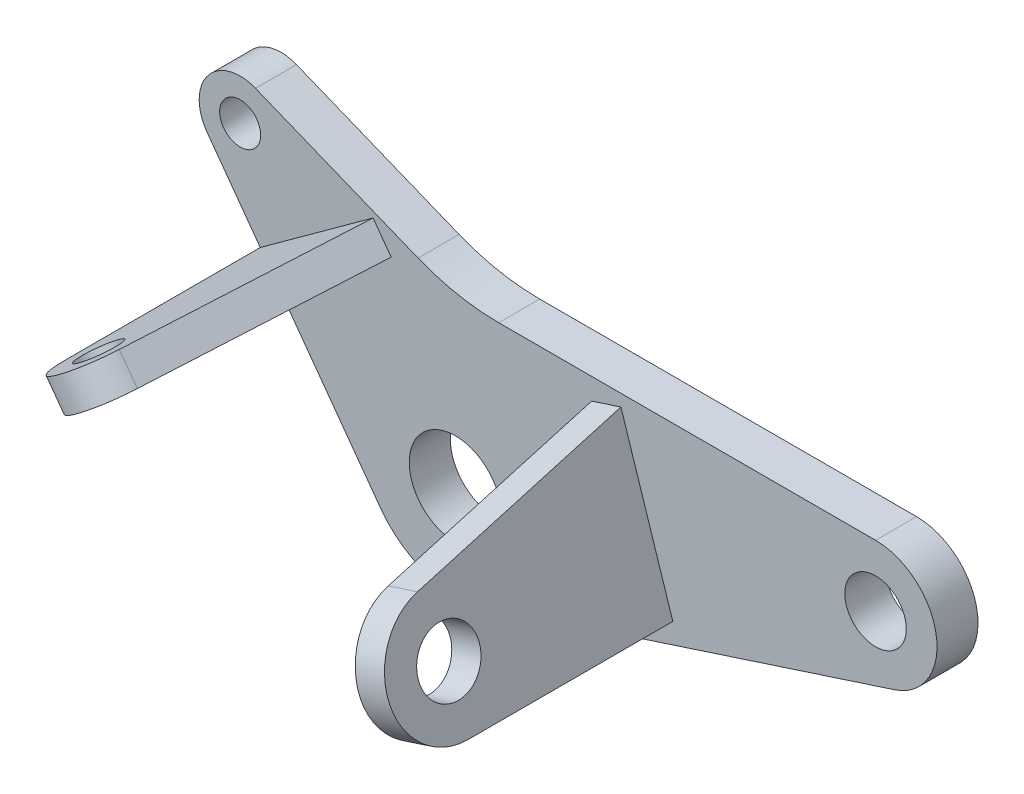
ISO-10303-21;
HEADER;
FILE_DESCRIPTION(('STEP AP214'),'2;1');
FILE_NAME('part.step','',(''),(''),'','','');
FILE_SCHEMA(('AUTOMOTIVE_DESIGN { 1 0 10303 214 1 1 1 1 }'));
ENDSEC;
DATA;
#1=APPLICATION_CONTEXT('core data for automotive mechanical design processes');
#2=APPLICATION_PROTOCOL_DEFINITION('international standard','automotive_design',2000,#1);
#3=PRODUCT_CONTEXT('',#1,'mechanical');
#4=PRODUCT('Part','Part','',(#3));
#5=PRODUCT_RELATED_PRODUCT_CATEGORY('part','',(#4));
#6=PRODUCT_DEFINITION_FORMATION('','',#4);
#7=PRODUCT_DEFINITION_CONTEXT('part definition',#1,'design');
#8=PRODUCT_DEFINITION('design','',#6,#7);
#9=PRODUCT_DEFINITION_SHAPE('','',#8);
#10=(LENGTH_UNIT() NAMED_UNIT(*) SI_UNIT(.MILLI.,.METRE.));
#11=(NAMED_UNIT(*) PLANE_ANGLE_UNIT() SI_UNIT($,.RADIAN.));
#12=(NAMED_UNIT(*) SI_UNIT($,.STERADIAN.) SOLID_ANGLE_UNIT());
#13=UNCERTAINTY_MEASURE_WITH_UNIT(LENGTH_MEASURE(1.E-05),#10,'distance_accuracy_value','');
#14=(GEOMETRIC_REPRESENTATION_CONTEXT(3) GLOBAL_UNCERTAINTY_ASSIGNED_CONTEXT((#13)) GLOBAL_UNIT_ASSIGNED_CONTEXT((#10,
#11,#12)) REPRESENTATION_CONTEXT('',''));
#15=CARTESIAN_POINT('',(0.,0.,0.));
#16=DIRECTION('',(0.,0.,1.));
#17=DIRECTION('',(1.,0.,0.));
#18=AXIS2_PLACEMENT_3D('',#15,#16,#17);
#19=CARTESIAN_POINT('',(-34.5470044766931,16.9264432674838,78.));
#20=DIRECTION('',(-0.587785252292472,0.809016994374948,0.));
#21=DIRECTION('',(-0.809016994374948,-0.587785252292472,0.));
#22=AXIS2_PLACEMENT_3D('',#19,#20,#21);
#23=PLANE('',#22);
#24=CARTESIAN_POINT('',(-28.0748685216935,21.6287252858236,46.));
#25=DIRECTION('',(-0.587785252292472,0.809016994374948,0.));
#26=DIRECTION('',(-0.809016994374948,-0.587785252292472,0.));
#27=AXIS2_PLACEMENT_3D('',#24,#25,#26);
#28=CIRCLE('',#27,4.00000000000001);
#29=CARTESIAN_POINT('',(-31.3109364991933,19.2775842766537,46.));
#30=VERTEX_POINT('',#29);
#31=EDGE_CURVE('E320',#30,#30,#28,.T.);
#32=ORIENTED_EDGE('',*,*,#31,.T.);
#33=EDGE_LOOP('',(#32));
#34=FACE_BOUND('',#33,.T.);
#35=CARTESIAN_POINT('',(-28.0748685216935,21.6287252858236,46.));
#36=DIRECTION('',(-0.587785252292472,0.809016994374948,0.));
#37=DIRECTION('',(-0.809016994374948,-0.587785252292472,0.));
#38=AXIS2_PLACEMENT_3D('',#35,#36,#37);
#39=CIRCLE('',#38,8.);
#40=CARTESIAN_POINT('',(-34.5470044766931,16.9264432674838,46.));
#41=VERTEX_POINT('',#40);
#42=CARTESIAN_POINT('',(-21.8534521372472,26.1488488735531,48.205098846536));
#43=VERTEX_POINT('',#42);
#44=EDGE_CURVE('E12',#41,#43,#39,.T.);
#45=ORIENTED_EDGE('',*,*,#44,.F.);
#46=DIRECTION('',(0.,0.,-1.));
#47=VECTOR('',#46,1.);
#48=CARTESIAN_POINT('',(-34.5470044766931,16.9264432674838,78.));
#49=LINE('',#48,#47);
#50=CARTESIAN_POINT('',(-34.5470044766931,16.9264432674838,8.));
#51=VERTEX_POINT('',#50);
#52=EDGE_CURVE('E213',#41,#51,#49,.T.);
#53=ORIENTED_EDGE('',*,*,#52,.T.);
#54=DIRECTION('',(0.809016994374948,0.587785252292472,0.));
#55=VECTOR('',#54,1.);
#56=CARTESIAN_POINT('',(-34.5470044766931,16.9264432674838,8.));
#57=LINE('',#56,#55);
#58=CARTESIAN_POINT('',(-12.5265973136636,32.9252055554185,8.));
#59=VERTEX_POINT('',#58);
#60=EDGE_CURVE('E225',#51,#59,#57,.T.);
#61=ORIENTED_EDGE('',*,*,#60,.T.);
#62=DIRECTION('',(-0.22299530514053,-0.162015572730127,0.961261695938318));
#63=VECTOR('',#62,1.);
#64=CARTESIAN_POINT('',(-29.204597873977,20.8079288662537,79.8935454419716));
#65=LINE('',#64,#63);
#66=EDGE_CURVE('E95',#59,#43,#65,.T.);
#67=ORIENTED_EDGE('',*,*,#66,.T.);
#68=EDGE_LOOP('',(#45,#53,#61,#67));
#69=FACE_BOUND('',#68,.T.);
#70=ADVANCED_FACE('F84',(#34,#69),#23,.F.);
#71=CARTESIAN_POINT('',(5.56230589874908,-17.1190172933128,8.));
#72=DIRECTION('',(-0.309016994374949,0.951056516295153,0.));
#73=DIRECTION('',(-0.951056516295153,-0.309016994374949,0.));
#74=AXIS2_PLACEMENT_3D('',#71,#72,#73);
#75=PLANE('',#74);
#76=DIRECTION('',(0.,0.,-1.));
#77=VECTOR('',#76,1.);
#78=CARTESIAN_POINT('',(85.7082039324994,8.92196355012698,8.));
#79=LINE('',#78,#77);
#80=CARTESIAN_POINT('',(85.7082039324994,8.92196355012698,8.));
#81=VERTEX_POINT('',#80);
#82=CARTESIAN_POINT('',(85.7082039324994,8.92196355012698,0.));
#83=VERTEX_POINT('',#82);
#84=EDGE_CURVE('E272',#81,#83,#79,.T.);
#85=ORIENTED_EDGE('',*,*,#84,.F.);
#86=DIRECTION('',(0.951056516295153,0.309016994374949,0.));
#87=VECTOR('',#86,1.);
#88=CARTESIAN_POINT('',(5.56230589874908,-17.1190172933128,8.));
#89=LINE('',#88,#87);
#90=CARTESIAN_POINT('',(5.56230589874908,-17.1190172933128,8.));
#91=VERTEX_POINT('',#90);
#92=EDGE_CURVE('E271',#91,#81,#89,.T.);
#93=ORIENTED_EDGE('',*,*,#92,.F.);
#94=DIRECTION('',(0.,0.,-1.));
#95=VECTOR('',#94,1.);
#96=CARTESIAN_POINT('',(5.56230589874908,-17.1190172933128,8.));
#97=LINE('',#96,#95);
#98=CARTESIAN_POINT('',(5.56230589874908,-17.1190172933128,0.));
#99=VERTEX_POINT('',#98);
#100=EDGE_CURVE('E292',#91,#99,#97,.T.);
#101=ORIENTED_EDGE('',*,*,#100,.T.);
#102=DIRECTION('',(0.951056516295153,0.309016994374949,0.));
#103=VECTOR('',#102,1.);
#104=CARTESIAN_POINT('',(5.56230589874908,-17.1190172933128,0.));
#105=LINE('',#104,#103);
#106=EDGE_CURVE('E256',#99,#83,#105,.T.);
#107=ORIENTED_EDGE('',*,*,#106,.T.);
#108=EDGE_LOOP('',(#85,#93,#101,#107));
#109=FACE_BOUND('',#108,.T.);
#110=ADVANCED_FACE('F384',(#109),#75,.F.);
#111=CARTESIAN_POINT('',(82.,20.3346417456688,8.));
#112=DIRECTION('',(0.,0.,1.));
#113=DIRECTION('',(1.,0.,0.));
#114=AXIS2_PLACEMENT_3D('',#111,#112,#113);
#115=PLANE('',#114);
#116=DIRECTION('',(-0.809016994374949,-0.587785252292471,0.));
#117=VECTOR('',#116,1.);
#118=CARTESIAN_POINT('',(-38.0737159904479,21.7805452337335,8.));
#119=LINE('',#118,#117);
#120=CARTESIAN_POINT('',(-16.0533088274185,37.7793075216682,8.));
#121=VERTEX_POINT('',#120);
#122=CARTESIAN_POINT('',(-38.0737159904479,21.7805452337335,8.));
#123=VERTEX_POINT('',#122);
#124=EDGE_CURVE('E217',#121,#123,#119,.T.);
#125=ORIENTED_EDGE('',*,*,#124,.F.);
#126=DIRECTION('',(-0.587785252292471,0.809016994374949,0.));
#127=VECTOR('',#126,1.);
#128=CARTESIAN_POINT('',(13.3359537872051,-2.67154219707923,8.));
#129=LINE('',#128,#127);
#130=EDGE_CURVE('E212',#59,#121,#129,.T.);
#131=ORIENTED_EDGE('',*,*,#130,.F.);
#132=ORIENTED_EDGE('',*,*,#60,.F.);
#133=DIRECTION('',(0.587785252292471,-0.809016994374949,0.));
#134=VECTOR('',#133,1.);
#135=CARTESIAN_POINT('',(-48.4721359549996,36.0927424744089,8.));
#136=LINE('',#135,#134);
#137=CARTESIAN_POINT('',(-14.5623058987491,-10.5801345412645,8.));
#138=VERTEX_POINT('',#137);
#139=EDGE_CURVE('E266',#51,#138,#136,.T.);
#140=ORIENTED_EDGE('',*,*,#139,.T.);
#141=CARTESIAN_POINT('',(0.,0.,8.));
#142=DIRECTION('',(0.,0.,1.));
#143=DIRECTION('',(1.,0.,0.));
#144=AXIS2_PLACEMENT_3D('',#141,#142,#143);
#145=CIRCLE('',#144,18.);
#146=EDGE_CURVE('E267',#138,#91,#145,.T.);
#147=ORIENTED_EDGE('',*,*,#146,.T.);
#148=ORIENTED_EDGE('',*,*,#92,.T.);
#149=CARTESIAN_POINT('',(82.,20.3346417456688,8.));
#150=DIRECTION('',(0.,0.,1.));
#151=DIRECTION('',(1.,0.,0.));
#152=AXIS2_PLACEMENT_3D('',#149,#150,#151);
#153=CIRCLE('',#152,12.);
#154=CARTESIAN_POINT('',(82.,32.3346417456688,8.));
#155=VERTEX_POINT('',#154);
#156=EDGE_CURVE('E255',#81,#155,#153,.T.);
#157=ORIENTED_EDGE('',*,*,#156,.T.);
#158=DIRECTION('',(-1.,0.,0.));
#159=VECTOR('',#158,1.);
#160=CARTESIAN_POINT('',(8.45989239638362,32.3346417456688,8.));
#161=LINE('',#160,#159);
#162=CARTESIAN_POINT('',(8.45989239638361,32.3346417456688,8.));
#163=VERTEX_POINT('',#162);
#164=EDGE_CURVE('E260',#155,#163,#161,.T.);
#165=ORIENTED_EDGE('',*,*,#164,.T.);
#166=CARTESIAN_POINT('',(8.45989239638362,74.3346417456688,8.));
#167=DIRECTION('',(0.,0.,-1.));
#168=DIRECTION('',(1.,0.,0.));
#169=AXIS2_PLACEMENT_3D('',#166,#167,#168);
#170=CIRCLE('',#169,42.);
#171=CARTESIAN_POINT('',(-7.27358452708473,35.3929198538638,8.));
#172=VERTEX_POINT('',#171);
#173=EDGE_CURVE('E257',#163,#172,#170,.T.);
#174=ORIENTED_EDGE('',*,*,#173,.T.);
#175=DIRECTION('',(-0.927183854566787,0.374606593415913,0.));
#176=VECTOR('',#175,1.);
#177=CARTESIAN_POINT('',(-39.0031472526727,48.212495329283,8.));
#178=LINE('',#177,#176);
#179=CARTESIAN_POINT('',(-39.0031472526727,48.212495329283,8.));
#180=VERTEX_POINT('',#179);
#181=EDGE_CURVE('E265',#172,#180,#178,.T.);
#182=ORIENTED_EDGE('',*,*,#181,.T.);
#183=CARTESIAN_POINT('',(-42.,40.7950244927487,8.));
#184=DIRECTION('',(0.,0.,1.));
#185=DIRECTION('',(1.,0.,0.));
#186=AXIS2_PLACEMENT_3D('',#183,#184,#185);
#187=CIRCLE('',#186,7.99999999999999);
#188=CARTESIAN_POINT('',(-48.4721359549996,36.0927424744089,8.));
#189=VERTEX_POINT('',#188);
#190=EDGE_CURVE('E262',#180,#189,#187,.T.);
#191=ORIENTED_EDGE('',*,*,#190,.T.);
#192=EDGE_CURVE('E270',#189,#123,#136,.T.);
#193=ORIENTED_EDGE('',*,*,#192,.T.);
#194=EDGE_LOOP('',(#125,#131,#132,#140,#147,#148,#157,#165,#174,#182,#191,#193));
#195=FACE_BOUND('',#194,.T.);
#196=DIRECTION('',(-0.309016994374949,0.951056516295153,0.));
#197=VECTOR('',#196,1.);
#198=CARTESIAN_POINT('',(43.6045665505552,-4.75833751831482,8.));
#199=LINE('',#198,#197);
#200=CARTESIAN_POINT('',(42.4340939331321,-1.15599321295721,8.));
#201=VERTEX_POINT('',#200);
#202=CARTESIAN_POINT('',(32.3074989935226,30.0104613203209,8.00000000000001));
#203=VERTEX_POINT('',#202);
#204=EDGE_CURVE('E355',#201,#203,#199,.T.);
#205=ORIENTED_EDGE('',*,*,#204,.F.);
#206=DIRECTION('',(0.951056516295153,0.309016994374949,0.));
#207=VECTOR('',#206,1.);
#208=CARTESIAN_POINT('',(-5.11873188162557,-16.6068429317046,8.));
#209=LINE('',#208,#207);
#210=CARTESIAN_POINT('',(36.7277548353611,-3.01009517920691,8.));
#211=VERTEX_POINT('',#210);
#212=EDGE_CURVE('E350',#211,#201,#209,.T.);
#213=ORIENTED_EDGE('',*,*,#212,.F.);
#214=DIRECTION('',(0.309016994374949,-0.951056516295153,0.));
#215=VECTOR('',#214,1.);
#216=CARTESIAN_POINT('',(37.8982274527843,-6.61243948456451,8.));
#217=LINE('',#216,#215);
#218=CARTESIAN_POINT('',(26.6011598957517,28.1563593540712,7.99999999999999));
#219=VERTEX_POINT('',#218);
#220=EDGE_CURVE('E234',#219,#211,#217,.T.);
#221=ORIENTED_EDGE('',*,*,#220,.F.);
#222=DIRECTION('',(-0.951056516295153,-0.309016994374949,0.));
#223=VECTOR('',#222,1.);
#224=CARTESIAN_POINT('',(26.6011598957517,28.1563593540712,8.));
#225=LINE('',#224,#223);
#226=EDGE_CURVE('E226',#203,#219,#225,.T.);
#227=ORIENTED_EDGE('',*,*,#226,.F.);
#228=EDGE_LOOP('',(#205,#213,#221,#227));
#229=FACE_BOUND('',#228,.T.);
#230=CARTESIAN_POINT('',(-42.,40.7950244927487,8.));
#231=DIRECTION('',(0.,0.,1.));
#232=DIRECTION('',(1.,0.,0.));
#233=AXIS2_PLACEMENT_3D('',#230,#231,#232);
#234=CIRCLE('',#233,4.00000000000001);
#235=CARTESIAN_POINT('',(-38.,40.7950244927487,8.));
#236=VERTEX_POINT('',#235);
#237=EDGE_CURVE('E245',#236,#236,#234,.T.);
#238=ORIENTED_EDGE('',*,*,#237,.F.);
#239=EDGE_LOOP('',(#238));
#240=FACE_BOUND('',#239,.T.);
#241=CARTESIAN_POINT('',(0.,0.,8.));
#242=DIRECTION('',(0.,0.,1.));
#243=DIRECTION('',(1.,0.,0.));
#244=AXIS2_PLACEMENT_3D('',#241,#242,#243);
#245=CIRCLE('',#244,9.);
#246=CARTESIAN_POINT('',(9.,0.,8.));
#247=VERTEX_POINT('',#246);
#248=EDGE_CURVE('E248',#247,#247,#245,.T.);
#249=ORIENTED_EDGE('',*,*,#248,.F.);
#250=EDGE_LOOP('',(#249));
#251=FACE_BOUND('',#250,.T.);
#252=CARTESIAN_POINT('',(82.,20.3346417456688,8.));
#253=DIRECTION('',(0.,0.,1.));
#254=DIRECTION('',(1.,0.,0.));
#255=AXIS2_PLACEMENT_3D('',#252,#253,#254);
#256=CIRCLE('',#255,6.);
#257=CARTESIAN_POINT('',(88.,20.3346417456688,8.));
#258=VERTEX_POINT('',#257);
#259=EDGE_CURVE('E231',#258,#258,#256,.T.);
#260=ORIENTED_EDGE('',*,*,#259,.F.);
#261=EDGE_LOOP('',(#260));
#262=FACE_BOUND('',#261,.T.);
#263=ADVANCED_FACE('F330',(#195,#229,#240,#251,#262),#115,.T.);
#264=CARTESIAN_POINT('',(82.,20.3346417456688,0.));
#265=DIRECTION('',(0.,0.,1.));
#266=DIRECTION('',(1.,0.,0.));
#267=AXIS2_PLACEMENT_3D('',#264,#265,#266);
#268=PLANE('',#267);
#269=CARTESIAN_POINT('',(82.,20.3346417456688,0.));
#270=DIRECTION('',(0.,0.,1.));
#271=DIRECTION('',(1.,0.,0.));
#272=AXIS2_PLACEMENT_3D('',#269,#270,#271);
#273=CIRCLE('',#272,12.);
#274=CARTESIAN_POINT('',(82.,32.3346417456688,0.));
#275=VERTEX_POINT('',#274);
#276=EDGE_CURVE('E253',#83,#275,#273,.T.);
#277=ORIENTED_EDGE('',*,*,#276,.F.);
#278=ORIENTED_EDGE('',*,*,#106,.F.);
#279=CARTESIAN_POINT('',(0.,0.,0.));
#280=DIRECTION('',(0.,0.,1.));
#281=DIRECTION('',(1.,0.,0.));
#282=AXIS2_PLACEMENT_3D('',#279,#280,#281);
#283=CIRCLE('',#282,18.);
#284=CARTESIAN_POINT('',(-14.5623058987491,-10.5801345412645,0.));
#285=VERTEX_POINT('',#284);
#286=EDGE_CURVE('E287',#285,#99,#283,.T.);
#287=ORIENTED_EDGE('',*,*,#286,.F.);
#288=DIRECTION('',(0.587785252292471,-0.809016994374949,0.));
#289=VECTOR('',#288,1.);
#290=CARTESIAN_POINT('',(-48.4721359549996,36.0927424744089,0.));
#291=LINE('',#290,#289);
#292=CARTESIAN_POINT('',(-48.4721359549996,36.0927424744089,0.));
#293=VERTEX_POINT('',#292);
#294=EDGE_CURVE('E282',#293,#285,#291,.T.);
#295=ORIENTED_EDGE('',*,*,#294,.F.);
#296=CARTESIAN_POINT('',(-42.,40.7950244927487,0.));
#297=DIRECTION('',(0.,0.,1.));
#298=DIRECTION('',(1.,0.,0.));
#299=AXIS2_PLACEMENT_3D('',#296,#297,#298);
#300=CIRCLE('',#299,7.99999999999999);
#301=CARTESIAN_POINT('',(-39.0031472526727,48.212495329283,0.));
#302=VERTEX_POINT('',#301);
#303=EDGE_CURVE('E285',#302,#293,#300,.T.);
#304=ORIENTED_EDGE('',*,*,#303,.F.);
#305=DIRECTION('',(-0.927183854566787,0.374606593415913,0.));
#306=VECTOR('',#305,1.);
#307=CARTESIAN_POINT('',(-39.0031472526727,48.212495329283,0.));
#308=LINE('',#307,#306);
#309=CARTESIAN_POINT('',(-7.27358452708473,35.3929198538638,0.));
#310=VERTEX_POINT('',#309);
#311=EDGE_CURVE('E278',#310,#302,#308,.T.);
#312=ORIENTED_EDGE('',*,*,#311,.F.);
#313=CARTESIAN_POINT('',(8.45989239638362,74.3346417456688,0.));
#314=DIRECTION('',(0.,0.,-1.));
#315=DIRECTION('',(1.,0.,0.));
#316=AXIS2_PLACEMENT_3D('',#313,#314,#315);
#317=CIRCLE('',#316,42.);
#318=CARTESIAN_POINT('',(8.45989239638361,32.3346417456688,0.));
#319=VERTEX_POINT('',#318);
#320=EDGE_CURVE('E279',#319,#310,#317,.T.);
#321=ORIENTED_EDGE('',*,*,#320,.F.);
#322=DIRECTION('',(-1.,0.,0.));
#323=VECTOR('',#322,1.);
#324=CARTESIAN_POINT('',(8.45989239638362,32.3346417456688,0.));
#325=LINE('',#324,#323);
#326=EDGE_CURVE('E277',#275,#319,#325,.T.);
#327=ORIENTED_EDGE('',*,*,#326,.F.);
#328=EDGE_LOOP('',(#277,#278,#287,#295,#304,#312,#321,#327));
#329=FACE_BOUND('',#328,.T.);
#330=CARTESIAN_POINT('',(0.,0.,0.));
#331=DIRECTION('',(0.,0.,1.));
#332=DIRECTION('',(1.,0.,0.));
#333=AXIS2_PLACEMENT_3D('',#330,#331,#332);
#334=CIRCLE('',#333,9.);
#335=CARTESIAN_POINT('',(9.,0.,0.));
#336=VERTEX_POINT('',#335);
#337=EDGE_CURVE('E244',#336,#336,#334,.T.);
#338=ORIENTED_EDGE('',*,*,#337,.T.);
#339=EDGE_LOOP('',(#338));
#340=FACE_BOUND('',#339,.T.);
#341=CARTESIAN_POINT('',(-42.,40.7950244927487,0.));
#342=DIRECTION('',(0.,0.,1.));
#343=DIRECTION('',(1.,0.,0.));
#344=AXIS2_PLACEMENT_3D('',#341,#342,#343);
#345=CIRCLE('',#344,4.00000000000001);
#346=CARTESIAN_POINT('',(-38.,40.7950244927487,0.));
#347=VERTEX_POINT('',#346);
#348=EDGE_CURVE('E236',#347,#347,#345,.T.);
#349=ORIENTED_EDGE('',*,*,#348,.T.);
#350=EDGE_LOOP('',(#349));
#351=FACE_BOUND('',#350,.T.);
#352=CARTESIAN_POINT('',(82.,20.3346417456688,0.));
#353=DIRECTION('',(0.,0.,1.));
#354=DIRECTION('',(1.,0.,0.));
#355=AXIS2_PLACEMENT_3D('',#352,#353,#354);
#356=CIRCLE('',#355,6.);
#357=CARTESIAN_POINT('',(88.,20.3346417456688,0.));
#358=VERTEX_POINT('',#357);
#359=EDGE_CURVE('E239',#358,#358,#356,.T.);
#360=ORIENTED_EDGE('',*,*,#359,.T.);
#361=EDGE_LOOP('',(#360));
#362=FACE_BOUND('',#361,.T.);
#363=ADVANCED_FACE('F412',(#329,#340,#351,#362),#268,.F.);
#364=CARTESIAN_POINT('',(82.,20.3346417456688,8.));
#365=DIRECTION('',(0.,0.,-1.));
#366=DIRECTION('',(-1.,0.,0.));
#367=AXIS2_PLACEMENT_3D('',#364,#365,#366);
#368=CYLINDRICAL_SURFACE('',#367,12.);
#369=ORIENTED_EDGE('',*,*,#276,.T.);
#370=DIRECTION('',(0.,0.,-1.));
#371=VECTOR('',#370,1.);
#372=CARTESIAN_POINT('',(82.,32.3346417456688,8.));
#373=LINE('',#372,#371);
#374=EDGE_CURVE('E310',#155,#275,#373,.T.);
#375=ORIENTED_EDGE('',*,*,#374,.F.);
#376=ORIENTED_EDGE('',*,*,#156,.F.);
#377=ORIENTED_EDGE('',*,*,#84,.T.);
#378=EDGE_LOOP('',(#369,#375,#376,#377));
#379=FACE_BOUND('',#378,.T.);
#380=ADVANCED_FACE('F88',(#379),#368,.T.);
#381=CARTESIAN_POINT('',(8.45989239638362,32.3346417456688,8.));
#382=DIRECTION('',(0.,-1.,0.));
#383=DIRECTION('',(1.,0.,0.));
#384=AXIS2_PLACEMENT_3D('',#381,#382,#383);
#385=PLANE('',#384);
#386=ORIENTED_EDGE('',*,*,#326,.T.);
#387=DIRECTION('',(0.,0.,-1.));
#388=VECTOR('',#387,1.);
#389=CARTESIAN_POINT('',(8.45989239638361,32.3346417456688,8.));
#390=LINE('',#389,#388);
#391=EDGE_CURVE('E308',#163,#319,#390,.T.);
#392=ORIENTED_EDGE('',*,*,#391,.F.);
#393=ORIENTED_EDGE('',*,*,#164,.F.);
#394=ORIENTED_EDGE('',*,*,#374,.T.);
#395=EDGE_LOOP('',(#386,#392,#393,#394));
#396=FACE_BOUND('',#395,.T.);
#397=ADVANCED_FACE('F429',(#396),#385,.F.);
#398=CARTESIAN_POINT('',(8.45989239638362,74.3346417456688,8.));
#399=DIRECTION('',(0.,0.,-1.));
#400=DIRECTION('',(-1.,0.,0.));
#401=AXIS2_PLACEMENT_3D('',#398,#399,#400);
#402=CYLINDRICAL_SURFACE('',#401,42.);
#403=ORIENTED_EDGE('',*,*,#320,.T.);
#404=DIRECTION('',(0.,0.,-1.));
#405=VECTOR('',#404,1.);
#406=CARTESIAN_POINT('',(-7.27358452708473,35.3929198538638,8.));
#407=LINE('',#406,#405);
#408=EDGE_CURVE('E303',#172,#310,#407,.T.);
#409=ORIENTED_EDGE('',*,*,#408,.F.);
#410=ORIENTED_EDGE('',*,*,#173,.F.);
#411=ORIENTED_EDGE('',*,*,#391,.T.);
#412=EDGE_LOOP('',(#403,#409,#410,#411));
#413=FACE_BOUND('',#412,.T.);
#414=ADVANCED_FACE('F430',(#413),#402,.F.);
#415=CARTESIAN_POINT('',(-39.0031472526727,48.212495329283,8.));
#416=DIRECTION('',(-0.374606593415913,-0.927183854566787,0.));
#417=DIRECTION('',(0.927183854566787,-0.374606593415913,0.));
#418=AXIS2_PLACEMENT_3D('',#415,#416,#417);
#419=PLANE('',#418);
#420=ORIENTED_EDGE('',*,*,#311,.T.);
#421=DIRECTION('',(0.,0.,-1.));
#422=VECTOR('',#421,1.);
#423=CARTESIAN_POINT('',(-39.0031472526727,48.212495329283,8.));
#424=LINE('',#423,#422);
#425=EDGE_CURVE('E299',#180,#302,#424,.T.);
#426=ORIENTED_EDGE('',*,*,#425,.F.);
#427=ORIENTED_EDGE('',*,*,#181,.F.);
#428=ORIENTED_EDGE('',*,*,#408,.T.);
#429=EDGE_LOOP('',(#420,#426,#427,#428));
#430=FACE_BOUND('',#429,.T.);
#431=ADVANCED_FACE('F421',(#430),#419,.F.);
#432=CARTESIAN_POINT('',(-42.,40.7950244927487,8.));
#433=DIRECTION('',(0.,0.,-1.));
#434=DIRECTION('',(-1.,0.,0.));
#435=AXIS2_PLACEMENT_3D('',#432,#433,#434);
#436=CYLINDRICAL_SURFACE('',#435,7.99999999999999);
#437=ORIENTED_EDGE('',*,*,#303,.T.);
#438=DIRECTION('',(0.,0.,-1.));
#439=VECTOR('',#438,1.);
#440=CARTESIAN_POINT('',(-48.4721359549996,36.0927424744089,8.));
#441=LINE('',#440,#439);
#442=EDGE_CURVE('E300',#189,#293,#441,.T.);
#443=ORIENTED_EDGE('',*,*,#442,.F.);
#444=ORIENTED_EDGE('',*,*,#190,.F.);
#445=ORIENTED_EDGE('',*,*,#425,.T.);
#446=EDGE_LOOP('',(#437,#443,#444,#445));
#447=FACE_BOUND('',#446,.T.);
#448=ADVANCED_FACE('F419',(#447),#436,.T.);
#449=CARTESIAN_POINT('',(-48.4721359549996,36.0927424744089,8.));
#450=DIRECTION('',(0.809016994374949,0.587785252292471,0.));
#451=DIRECTION('',(-0.587785252292471,0.809016994374949,0.));
#452=AXIS2_PLACEMENT_3D('',#449,#450,#451);
#453=PLANE('',#452);
#454=ORIENTED_EDGE('',*,*,#52,.F.);
#455=DIRECTION('',(-0.587785252292471,0.809016994374949,0.));
#456=VECTOR('',#455,1.);
#457=CARTESIAN_POINT('',(-8.68445337582437,-18.670304485014,46.));
#458=LINE('',#457,#456);
#459=CARTESIAN_POINT('',(-38.0737159904479,21.7805452337335,46.));
#460=VERTEX_POINT('',#459);
#461=EDGE_CURVE('E200',#41,#460,#458,.T.);
#462=ORIENTED_EDGE('',*,*,#461,.T.);
#463=DIRECTION('',(0.,0.,-1.));
#464=VECTOR('',#463,1.);
#465=CARTESIAN_POINT('',(-38.0737159904479,21.7805452337335,78.));
#466=LINE('',#465,#464);
#467=EDGE_CURVE('E209',#460,#123,#466,.T.);
#468=ORIENTED_EDGE('',*,*,#467,.T.);
#469=ORIENTED_EDGE('',*,*,#192,.F.);
#470=ORIENTED_EDGE('',*,*,#442,.T.);
#471=ORIENTED_EDGE('',*,*,#294,.T.);
#472=DIRECTION('',(0.,0.,-1.));
#473=VECTOR('',#472,1.);
#474=CARTESIAN_POINT('',(-14.5623058987491,-10.5801345412645,8.));
#475=LINE('',#474,#473);
#476=EDGE_CURVE('E294',#138,#285,#475,.T.);
#477=ORIENTED_EDGE('',*,*,#476,.F.);
#478=ORIENTED_EDGE('',*,*,#139,.F.);
#479=EDGE_LOOP('',(#454,#462,#468,#469,#470,#471,#477,#478));
#480=FACE_BOUND('',#479,.T.);
#481=ADVANCED_FACE('F208',(#480),#453,.F.);
#482=CARTESIAN_POINT('',(0.,0.,8.));
#483=DIRECTION('',(0.,0.,-1.));
#484=DIRECTION('',(-1.,0.,0.));
#485=AXIS2_PLACEMENT_3D('',#482,#483,#484);
#486=CYLINDRICAL_SURFACE('',#485,18.);
#487=ORIENTED_EDGE('',*,*,#286,.T.);
#488=ORIENTED_EDGE('',*,*,#100,.F.);
#489=ORIENTED_EDGE('',*,*,#146,.F.);
#490=ORIENTED_EDGE('',*,*,#476,.T.);
#491=EDGE_LOOP('',(#487,#488,#489,#490));
#492=FACE_BOUND('',#491,.T.);
#493=ADVANCED_FACE('F406',(#492),#486,.T.);
#494=CARTESIAN_POINT('',(0.,0.,8.));
#495=DIRECTION('',(0.,0.,-1.));
#496=DIRECTION('',(-1.,0.,0.));
#497=AXIS2_PLACEMENT_3D('',#494,#495,#496);
#498=CYLINDRICAL_SURFACE('',#497,9.);
#499=ORIENTED_EDGE('',*,*,#248,.T.);
#500=EDGE_LOOP('',(#499));
#501=FACE_BOUND('',#500,.T.);
#502=ORIENTED_EDGE('',*,*,#337,.F.);
#503=EDGE_LOOP('',(#502));
#504=FACE_BOUND('',#503,.T.);
#505=ADVANCED_FACE('F404',(#501,#504),#498,.F.);
#506=CARTESIAN_POINT('',(-42.,40.7950244927487,8.));
#507=DIRECTION('',(0.,0.,-1.));
#508=DIRECTION('',(-1.,0.,0.));
#509=AXIS2_PLACEMENT_3D('',#506,#507,#508);
#510=CYLINDRICAL_SURFACE('',#509,4.00000000000001);
#511=ORIENTED_EDGE('',*,*,#237,.T.);
#512=EDGE_LOOP('',(#511));
#513=FACE_BOUND('',#512,.T.);
#514=ORIENTED_EDGE('',*,*,#348,.F.);
#515=EDGE_LOOP('',(#514));
#516=FACE_BOUND('',#515,.T.);
#517=ADVANCED_FACE('F396',(#513,#516),#510,.F.);
#518=CARTESIAN_POINT('',(82.,20.3346417456688,8.));
#519=DIRECTION('',(0.,0.,-1.));
#520=DIRECTION('',(-1.,0.,0.));
#521=AXIS2_PLACEMENT_3D('',#518,#519,#520);
#522=CYLINDRICAL_SURFACE('',#521,6.);
#523=ORIENTED_EDGE('',*,*,#259,.T.);
#524=EDGE_LOOP('',(#523));
#525=FACE_BOUND('',#524,.T.);
#526=ORIENTED_EDGE('',*,*,#359,.F.);
#527=EDGE_LOOP('',(#526));
#528=FACE_BOUND('',#527,.T.);
#529=ADVANCED_FACE('F400',(#525,#528),#522,.F.);
#530=CARTESIAN_POINT('',(-38.0737159904479,21.7805452337335,78.));
#531=DIRECTION('',(0.587785252292471,-0.809016994374949,0.));
#532=DIRECTION('',(0.809016994374949,0.587785252292471,0.));
#533=AXIS2_PLACEMENT_3D('',#530,#531,#532);
#534=PLANE('',#533);
#535=CARTESIAN_POINT('',(-31.6015800354483,26.4828272520733,46.));
#536=DIRECTION('',(-0.587785252292471,0.809016994374949,0.));
#537=DIRECTION('',(-0.809016994374949,-0.587785252292472,0.));
#538=AXIS2_PLACEMENT_3D('',#535,#536,#537);
#539=CIRCLE('',#538,4.00000000000001);
#540=CARTESIAN_POINT('',(-34.8376480129481,24.1316862429034,46.));
#541=VERTEX_POINT('',#540);
#542=EDGE_CURVE('E319',#541,#541,#539,.T.);
#543=ORIENTED_EDGE('',*,*,#542,.F.);
#544=EDGE_LOOP('',(#543));
#545=FACE_BOUND('',#544,.T.);
#546=ORIENTED_EDGE('',*,*,#467,.F.);
#547=CARTESIAN_POINT('',(-31.6015800354483,26.4828272520732,46.));
#548=DIRECTION('',(-0.587785252292471,0.809016994374949,0.));
#549=DIRECTION('',(-0.809016994374949,-0.587785252292472,0.));
#550=AXIS2_PLACEMENT_3D('',#547,#548,#549);
#551=CIRCLE('',#550,8.);
#552=CARTESIAN_POINT('',(-25.3801636510021,31.0029508398028,48.205098846536));
#553=VERTEX_POINT('',#552);
#554=EDGE_CURVE('E198',#460,#553,#551,.T.);
#555=ORIENTED_EDGE('',*,*,#554,.T.);
#556=DIRECTION('',(-0.22299530514053,-0.162015572730127,0.961261695938318));
#557=VECTOR('',#556,1.);
#558=CARTESIAN_POINT('',(-14.9050904088559,38.6135370341929,3.05039631377227));
#559=LINE('',#558,#557);
#560=EDGE_CURVE('E204',#121,#553,#559,.T.);
#561=ORIENTED_EDGE('',*,*,#560,.F.);
#562=ORIENTED_EDGE('',*,*,#124,.T.);
#563=EDGE_LOOP('',(#546,#555,#561,#562));
#564=FACE_BOUND('',#563,.T.);
#565=ADVANCED_FACE('F216',(#545,#564),#534,.F.);
#566=CARTESIAN_POINT('',(37.8982274527843,-6.61243948456451,78.));
#567=DIRECTION('',(0.951056516295153,0.309016994374949,0.));
#568=DIRECTION('',(-0.309016994374949,0.951056516295153,0.));
#569=AXIS2_PLACEMENT_3D('',#566,#567,#568);
#570=PLANE('',#569);
#571=CARTESIAN_POINT('',(33.0195509028618,8.40258301633494,48.));
#572=DIRECTION('',(0.951056516295153,0.309016994374949,0.));
#573=DIRECTION('',(-0.309016994374949,0.951056516295153,0.));
#574=AXIS2_PLACEMENT_3D('',#571,#572,#573);
#575=CIRCLE('',#574,5.99999999999999);
#576=CARTESIAN_POINT('',(31.1654489366121,14.1089221141058,48.));
#577=VERTEX_POINT('',#576);
#578=EDGE_CURVE('E219',#577,#577,#575,.T.);
#579=ORIENTED_EDGE('',*,*,#578,.T.);
#580=EDGE_LOOP('',(#579));
#581=FACE_BOUND('',#580,.T.);
#582=ORIENTED_EDGE('',*,*,#220,.T.);
#583=DIRECTION('',(0.,0.,1.));
#584=VECTOR('',#583,1.);
#585=CARTESIAN_POINT('',(36.7277548353611,-3.01009517920691,78.));
#586=LINE('',#585,#584);
#587=CARTESIAN_POINT('',(36.7277548353611,-3.01009517920691,48.));
#588=VERTEX_POINT('',#587);
#589=EDGE_CURVE('E314',#211,#588,#586,.T.);
#590=ORIENTED_EDGE('',*,*,#589,.T.);
#591=CARTESIAN_POINT('',(33.0195509028618,8.40258301633493,48.));
#592=DIRECTION('',(0.951056516295153,0.309016994374949,0.));
#593=DIRECTION('',(-0.309016994374949,0.951056516295153,0.));
#594=AXIS2_PLACEMENT_3D('',#591,#592,#593);
#595=CIRCLE('',#594,12.);
#596=CARTESIAN_POINT('',(29.3923801232558,19.5658668112512,50.4949402898132));
#597=VERTEX_POINT('',#596);
#598=EDGE_CURVE('E223',#597,#588,#595,.T.);
#599=ORIENTED_EDGE('',*,*,#598,.F.);
#600=DIRECTION('',(0.0642482457919188,-0.197735768366177,0.978147600733805));
#601=VECTOR('',#600,1.);
#602=CARTESIAN_POINT('',(31.4886000216541,13.1143653396516,82.4088460930852));
#603=LINE('',#602,#601);
#604=EDGE_CURVE('E315',#219,#597,#603,.T.);
#605=ORIENTED_EDGE('',*,*,#604,.F.);
#606=EDGE_LOOP('',(#582,#590,#599,#605));
#607=FACE_BOUND('',#606,.T.);
#608=ADVANCED_FACE('F365',(#581,#607),#570,.F.);
#609=CARTESIAN_POINT('',(43.6045665505552,-4.75833751831482,78.));
#610=DIRECTION('',(-0.951056516295153,-0.309016994374949,0.));
#611=DIRECTION('',(0.309016994374949,-0.951056516295153,0.));
#612=AXIS2_PLACEMENT_3D('',#609,#610,#611);
#613=PLANE('',#612);
#614=CARTESIAN_POINT('',(38.7258900006327,10.2566849825846,48.));
#615=DIRECTION('',(0.951056516295153,0.309016994374949,0.));
#616=DIRECTION('',(-0.309016994374949,0.951056516295153,0.));
#617=AXIS2_PLACEMENT_3D('',#614,#615,#616);
#618=CIRCLE('',#617,5.99999999999999);
#619=CARTESIAN_POINT('',(36.871788034383,15.9630240803555,48.));
#620=VERTEX_POINT('',#619);
#621=EDGE_CURVE('E317',#620,#620,#618,.T.);
#622=ORIENTED_EDGE('',*,*,#621,.F.);
#623=EDGE_LOOP('',(#622));
#624=FACE_BOUND('',#623,.T.);
#625=ORIENTED_EDGE('',*,*,#204,.T.);
#626=DIRECTION('',(0.0642482457919188,-0.197735768366177,0.978147600733805));
#627=VECTOR('',#626,1.);
#628=CARTESIAN_POINT('',(32.0526429510887,30.7948275664694,4.11994345734157));
#629=LINE('',#628,#627);
#630=CARTESIAN_POINT('',(35.0987192210268,21.4199687775009,50.4949402898132));
#631=VERTEX_POINT('',#630);
#632=EDGE_CURVE('E339',#203,#631,#629,.T.);
#633=ORIENTED_EDGE('',*,*,#632,.T.);
#634=CARTESIAN_POINT('',(38.7258900006327,10.2566849825846,48.));
#635=DIRECTION('',(0.951056516295153,0.309016994374949,0.));
#636=DIRECTION('',(-0.309016994374949,0.951056516295153,0.));
#637=AXIS2_PLACEMENT_3D('',#634,#635,#636);
#638=CIRCLE('',#637,12.);
#639=CARTESIAN_POINT('',(42.4340939331321,-1.15599321295722,48.));
#640=VERTEX_POINT('',#639);
#641=EDGE_CURVE('E340',#631,#640,#638,.T.);
#642=ORIENTED_EDGE('',*,*,#641,.T.);
#643=DIRECTION('',(0.,0.,1.));
#644=VECTOR('',#643,1.);
#645=CARTESIAN_POINT('',(42.4340939331321,-1.15599321295721,0.));
#646=LINE('',#645,#644);
#647=EDGE_CURVE('E106',#201,#640,#646,.T.);
#648=ORIENTED_EDGE('',*,*,#647,.F.);
#649=EDGE_LOOP('',(#625,#633,#642,#648));
#650=FACE_BOUND('',#649,.T.);
#651=ADVANCED_FACE('F366',(#624,#650),#613,.F.);
#652=CARTESIAN_POINT('',(-5.11873188162557,-16.6068429317046,0.));
#653=DIRECTION('',(-0.309016994374949,0.951056516295153,0.));
#654=DIRECTION('',(-0.951056516295153,-0.309016994374949,0.));
#655=AXIS2_PLACEMENT_3D('',#652,#653,#654);
#656=PLANE('',#655);
#657=ORIENTED_EDGE('',*,*,#212,.T.);
#658=ORIENTED_EDGE('',*,*,#647,.T.);
#659=DIRECTION('',(0.951056516295153,0.309016994374949,0.));
#660=VECTOR('',#659,1.);
#661=CARTESIAN_POINT('',(-5.11873188162557,-16.6068429317046,48.));
#662=LINE('',#661,#660);
#663=EDGE_CURVE('E341',#588,#640,#662,.T.);
#664=ORIENTED_EDGE('',*,*,#663,.F.);
#665=ORIENTED_EDGE('',*,*,#589,.F.);
#666=EDGE_LOOP('',(#657,#658,#664,#665));
#667=FACE_BOUND('',#666,.T.);
#668=ADVANCED_FACE('F370',(#667),#656,.F.);
#669=CARTESIAN_POINT('',(-15.500182863669,15.343977847722,4.11994345734157));
#670=DIRECTION('',(-0.302264231633828,0.930273649576355,0.207911690817763));
#671=DIRECTION('',(-0.951056516295153,-0.309016994374949,0.));
#672=AXIS2_PLACEMENT_3D('',#669,#670,#671);
#673=PLANE('',#672);
#674=ORIENTED_EDGE('',*,*,#604,.T.);
#675=DIRECTION('',(0.951056516295153,0.309016994374949,0.));
#676=VECTOR('',#675,1.);
#677=CARTESIAN_POINT('',(-12.4541065937309,5.96911905875346,50.4949402898132));
#678=LINE('',#677,#676);
#679=EDGE_CURVE('E344',#597,#631,#678,.T.);
#680=ORIENTED_EDGE('',*,*,#679,.T.);
#681=ORIENTED_EDGE('',*,*,#632,.F.);
#682=ORIENTED_EDGE('',*,*,#226,.T.);
#683=EDGE_LOOP('',(#674,#680,#681,#682));
#684=FACE_BOUND('',#683,.T.);
#685=ADVANCED_FACE('F359',(#684),#673,.T.);
#686=CARTESIAN_POINT('',(-8.82693581412496,-5.1941647361628,48.));
#687=DIRECTION('',(0.951056516295153,0.309016994374949,0.));
#688=DIRECTION('',(-0.309016994374949,0.951056516295153,0.));
#689=AXIS2_PLACEMENT_3D('',#686,#687,#688);
#690=CYLINDRICAL_SURFACE('',#689,12.);
#691=ORIENTED_EDGE('',*,*,#598,.T.);
#692=ORIENTED_EDGE('',*,*,#663,.T.);
#693=ORIENTED_EDGE('',*,*,#641,.F.);
#694=ORIENTED_EDGE('',*,*,#679,.F.);
#695=EDGE_LOOP('',(#691,#692,#693,#694));
#696=FACE_BOUND('',#695,.T.);
#697=ADVANCED_FACE('F371',(#696),#690,.T.);
#698=CARTESIAN_POINT('',(-8.82693581412496,-5.1941647361628,48.));
#699=DIRECTION('',(0.951056516295153,0.309016994374949,0.));
#700=DIRECTION('',(-0.309016994374949,0.951056516295153,0.));
#701=AXIS2_PLACEMENT_3D('',#698,#699,#700);
#702=CYLINDRICAL_SURFACE('',#701,5.99999999999999);
#703=ORIENTED_EDGE('',*,*,#621,.T.);
#704=EDGE_LOOP('',(#703));
#705=FACE_BOUND('',#704,.T.);
#706=ORIENTED_EDGE('',*,*,#578,.F.);
#707=EDGE_LOOP('',(#706));
#708=FACE_BOUND('',#707,.T.);
#709=ADVANCED_FACE('F373',(#705,#708),#702,.F.);
#710=CARTESIAN_POINT('',(-2.21231742082477,-13.9680224666742,46.));
#711=DIRECTION('',(-0.587785252292471,0.809016994374949,0.));
#712=DIRECTION('',(-0.809016994374949,-0.587785252292471,0.));
#713=AXIS2_PLACEMENT_3D('',#710,#711,#712);
#714=CYLINDRICAL_SURFACE('',#713,4.00000000000001);
#715=ORIENTED_EDGE('',*,*,#542,.T.);
#716=EDGE_LOOP('',(#715));
#717=FACE_BOUND('',#716,.T.);
#718=ORIENTED_EDGE('',*,*,#31,.F.);
#719=EDGE_LOOP('',(#718));
#720=FACE_BOUND('',#719,.T.);
#721=ADVANCED_FACE('F377',(#717,#720),#714,.F.);
#722=CARTESIAN_POINT('',(-2.21231742082476,-13.9680224666742,46.));
#723=DIRECTION('',(-0.587785252292471,0.809016994374949,0.));
#724=DIRECTION('',(-0.809016994374949,-0.587785252292471,0.));
#725=AXIS2_PLACEMENT_3D('',#722,#723,#724);
#726=CYLINDRICAL_SURFACE('',#725,8.);
#727=ORIENTED_EDGE('',*,*,#44,.T.);
#728=DIRECTION('',(-0.587785252292471,0.809016994374949,0.));
#729=VECTOR('',#728,1.);
#730=CARTESIAN_POINT('',(4.0090989636215,-9.44789887894464,48.205098846536));
#731=LINE('',#730,#729);
#732=EDGE_CURVE('E97',#43,#553,#731,.T.);
#733=ORIENTED_EDGE('',*,*,#732,.T.);
#734=ORIENTED_EDGE('',*,*,#554,.F.);
#735=ORIENTED_EDGE('',*,*,#461,.F.);
#736=EDGE_LOOP('',(#727,#733,#734,#735));
#737=FACE_BOUND('',#736,.T.);
#738=ADVANCED_FACE('F196',(#737),#726,.T.);
#739=CARTESIAN_POINT('',(14.4841722057677,-1.83731268455449,3.05039631377227));
#740=DIRECTION('',(-0.777677048055784,-0.565015448466193,-0.275637355817003));
#741=DIRECTION('',(0.587785252292471,-0.809016994374949,0.));
#742=AXIS2_PLACEMENT_3D('',#739,#740,#741);
#743=PLANE('',#742);
#744=ORIENTED_EDGE('',*,*,#130,.T.);
#745=ORIENTED_EDGE('',*,*,#560,.T.);
#746=ORIENTED_EDGE('',*,*,#732,.F.);
#747=ORIENTED_EDGE('',*,*,#66,.F.);
#748=EDGE_LOOP('',(#744,#745,#746,#747));
#749=FACE_BOUND('',#748,.T.);
#750=ADVANCED_FACE('F324',(#749),#743,.F.);
#751=CLOSED_SHELL('',(#70,#110,#263,#363,#380,#397,#414,#431,#448,#481,#493,#505,#517,#529,#565,
#608,#651,#668,#685,#697,#709,#721,#738,#750));
#752=MANIFOLD_SOLID_BREP('B2',#751);
#753=ADVANCED_BREP_SHAPE_REPRESENTATION('',(#18,#752),#14);
#754=SHAPE_DEFINITION_REPRESENTATION(#9,#753);
ENDSEC;
END-ISO-10303-21;
